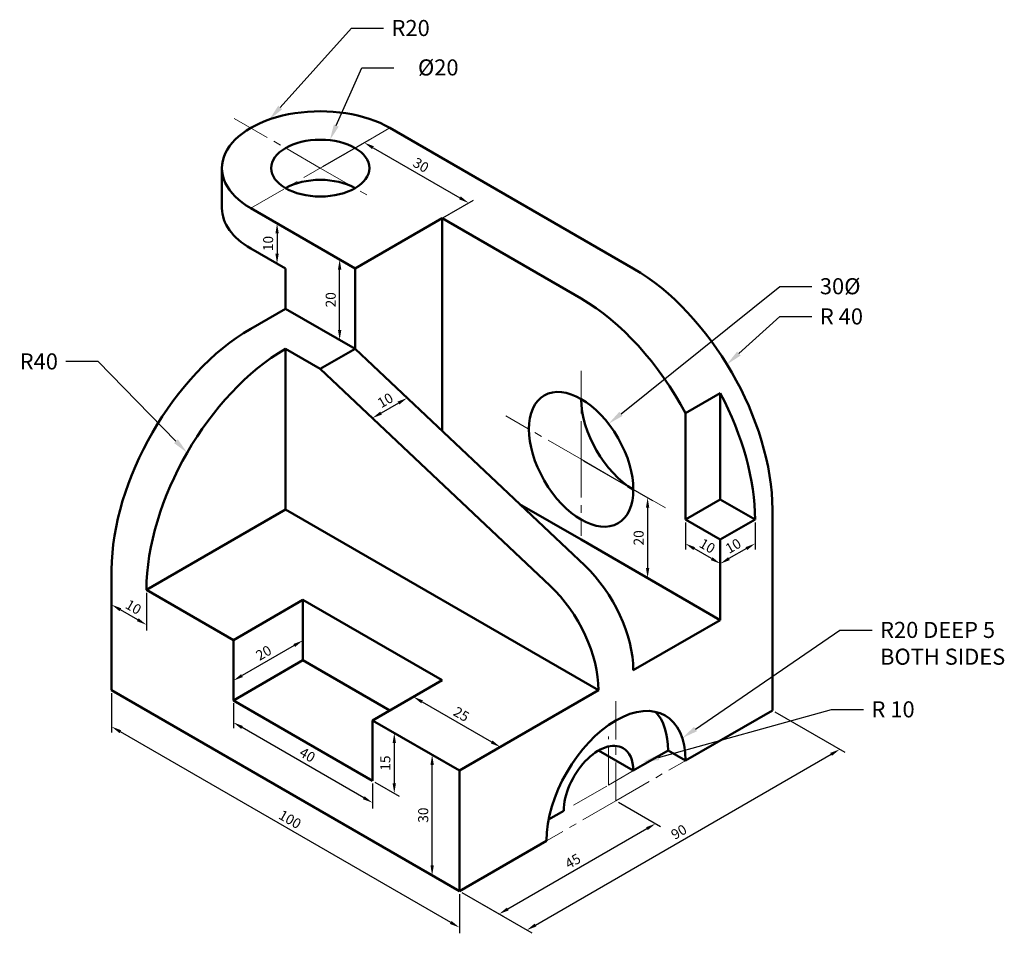
# Model space of a CAD drawing. Units: millimetres. Extents: x 1794 to 2039, y 1624 to 1851.
import ezdxf
from ezdxf import colors
from ezdxf.entities.mleader import LeaderData, LeaderLine
from ezdxf.math import Vec2, Vec3

# ---------------------------------------------------------------- set-up
doc = ezdxf.new("R2010")
doc.units = ezdxf.units.MM
doc.linetypes.add('CENTER', pattern=[50.8, 31.75, -6.35, 6.35, -6.35])
for name, color, linetype, lineweight in [('M-CNTR', 1, 'CENTER', 18), ('M-DIMS', 2, 'Continuous', 25), ('M-OUTL', 7, 'Continuous', 50)]:
    doc.layers.add(name, color=color, linetype=linetype, lineweight=lineweight)
doc.styles.get("Standard").update_dxf_attribs({"font": 'arial.ttf'})
doc.dimstyles.new('ISO-25', dxfattribs={"dimtxt": 2.5, "dimasz": 2.5, "dimexe": 1.25, "dimexo": 0.625, "dimtad": 1, "dimtxsty": 'Standard', "dimcen": 2.5, "dimadec": 0, "dimazin": 0, "dimtfac": 1, "dimtmove": 0, "dimatfit": 3, "dimfxl": 1, "dimarcsym": 0})

# ---------------------------------------------------------------- blocks, each defined once
blk = doc.blocks.new('*D1')
at = {"layer": 'Defpoints', "color": 0, "transparency": 16777216}
for p in [(1942.35, 1657.01), (1903.38, 1634.51), (1913.24, 1628.81)]:
    blk.add_point(p, dxfattribs=at)
at = {"layer": 'M-DIMS', "color": 0, "lineweight": -2, "transparency": 16777216}
for p, q in [((1942.97, 1656.65), (1953.46, 1650.59)), ((1950.05, 1650.06), (1915.41, 1630.06)), ((1904, 1634.15), (1914.49, 1628.09))]:
    blk.add_line(p, q, dxfattribs=at)
at = {"layer": 'M-DIMS', "color": 0, "transparency": 16777216}
for points in [[(1949.84, 1650.42), (1950.26, 1649.7), (1952.21, 1651.31)], [(1915.2, 1630.42), (1915.62, 1629.7), (1913.24, 1628.81)]]:
    blk.add_solid(points, dxfattribs=at)
at = {"layer": 'M-DIMS', "color": 0, "transparency": 16777216, "insert": (1931.78, 1641.71), "char_height": 2.5, "attachment_point": 5, "rotation": 30}
blk.add_mtext('45', dxfattribs=at)
blk = doc.blocks.new('*D2')
at = {"layer": 'Defpoints', "color": 0, "transparency": 16777216}
for p in [(1816.77, 1684.51), (1816.77, 1675.46), (1903.38, 1634.51)]:
    blk.add_point(p, dxfattribs=at)
at = {"layer": 'M-DIMS', "color": 0, "lineweight": -2, "transparency": 16777216}
for p, q in [((1816.77, 1683.79), (1816.77, 1674.01)), ((1901.21, 1626.71), (1818.94, 1674.21)), ((1903.38, 1633.79), (1903.38, 1624.01))]:
    blk.add_line(p, q, dxfattribs=at)
at = {"layer": 'M-DIMS', "color": 0, "transparency": 16777216}
for points in [[(1819.15, 1674.57), (1818.73, 1673.85), (1816.77, 1675.46)], [(1901.42, 1627.07), (1901, 1626.35), (1903.38, 1625.46)]]:
    blk.add_solid(points, dxfattribs=at)
at = {"layer": 'M-DIMS', "color": 0, "transparency": 16777216, "insert": (1861.03, 1652.1), "char_height": 2.5, "attachment_point": 5, "rotation": 330}
blk.add_mtext('100', dxfattribs=at)
blk = doc.blocks.new('*D3')
at = {"layer": 'Defpoints', "color": 0, "transparency": 16777216}
for p in [(1881.73, 1677.01), (1881.73, 1662.01), (1887.15, 1658.88)]:
    blk.add_point(p, dxfattribs=at)
at = {"layer": 'M-DIMS', "color": 0, "lineweight": -2, "transparency": 16777216}
for p, q in [((1882.35, 1676.65), (1888.4, 1673.16)), ((1887.15, 1671.38), (1887.15, 1661.38)), ((1882.35, 1661.65), (1888.4, 1658.16))]:
    blk.add_line(p, q, dxfattribs=at)
at = {"layer": 'M-DIMS', "color": 0, "transparency": 16777216}
for points in [[(1886.73, 1671.38), (1887.57, 1671.38), (1887.15, 1673.88)], [(1886.73, 1661.38), (1887.57, 1661.38), (1887.15, 1658.88)]]:
    blk.add_solid(points, dxfattribs=at)
at = {"layer": 'M-DIMS', "color": 0, "transparency": 16777216, "insert": (1885.25, 1666.38), "char_height": 2.5, "attachment_point": 5, "rotation": 90}
blk.add_mtext('15', dxfattribs=at)
blk = doc.blocks.new('*D4')
at = {"layer": 'Defpoints', "color": 0, "transparency": 16777216}
for p in [(1847.08, 1682.01), (1847.08, 1676.51), (1881.73, 1662.01)]:
    blk.add_point(p, dxfattribs=at)
at = {"layer": 'M-DIMS', "color": 0, "lineweight": -2, "transparency": 16777216}
for p, q in [((1847.08, 1681.29), (1847.08, 1675.07)), ((1879.56, 1657.76), (1849.25, 1675.26)), ((1881.73, 1661.29), (1881.73, 1655.07))]:
    blk.add_line(p, q, dxfattribs=at)
at = {"layer": 'M-DIMS', "color": 0, "transparency": 16777216}
for points in [[(1849.46, 1675.62), (1849.04, 1674.9), (1847.08, 1676.51)], [(1879.77, 1658.12), (1879.35, 1657.4), (1881.73, 1656.51)]]:
    blk.add_solid(points, dxfattribs=at)
at = {"layer": 'M-DIMS', "color": 0, "transparency": 16777216, "insert": (1865.36, 1668.16), "char_height": 2.5, "attachment_point": 5, "rotation": 330}
blk.add_mtext('40', dxfattribs=at)
blk = doc.blocks.new('*D5')
at = {"layer": 'Defpoints', "color": 0, "transparency": 16777216}
for p in [(1981.32, 1679.51), (1998.1, 1669.82), (1903.38, 1634.51)]:
    blk.add_point(p, dxfattribs=at)
at = {"layer": 'M-DIMS', "color": 0, "lineweight": -2, "transparency": 16777216}
for p, q in [((1981.94, 1679.15), (1999.35, 1669.1)), ((1922.32, 1626.07), (1995.93, 1668.57)), ((1904, 1634.15), (1921.4, 1624.1))]:
    blk.add_line(p, q, dxfattribs=at)
at = {"layer": 'M-DIMS', "color": 0, "transparency": 16777216}
for points in [[(1995.72, 1668.93), (1996.14, 1668.21), (1998.1, 1669.82)], [(1922.11, 1626.43), (1922.53, 1625.71), (1920.15, 1624.82)]]:
    blk.add_solid(points, dxfattribs=at)
at = {"layer": 'M-DIMS', "color": 0, "transparency": 16777216, "insert": (1958.18, 1648.97), "char_height": 2.5, "attachment_point": 5, "rotation": 30}
blk.add_mtext('90', dxfattribs=at)
blk = doc.blocks.new('*D6')
at = {"layer": 'Defpoints', "color": 0, "transparency": 16777216}
for p in [(1873.55, 1791.73), (1877.4, 1789.51), (1877.4, 1769.51)]:
    blk.add_point(p, dxfattribs=at)
at = {"layer": 'M-DIMS', "color": 0, "lineweight": -2, "transparency": 16777216}
for p, q in [((1876.77, 1789.87), (1872.3, 1792.45)), ((1873.55, 1774.23), (1873.55, 1789.23)), ((1876.77, 1769.87), (1872.3, 1772.45))]:
    blk.add_line(p, q, dxfattribs=at)
at = {"layer": 'M-DIMS', "color": 0, "transparency": 16777216}
for points in [[(1873.13, 1789.23), (1873.97, 1789.23), (1873.55, 1791.73)], [(1873.13, 1774.23), (1873.97, 1774.23), (1873.55, 1771.73)]]:
    blk.add_solid(points, dxfattribs=at)
at = {"layer": 'M-DIMS', "color": 0, "transparency": 16777216, "insert": (1871.65, 1781.73), "char_height": 2.5, "attachment_point": 5, "rotation": 90}
blk.add_mtext('20', dxfattribs=at)
blk = doc.blocks.new('*D7')
at = {"layer": 'Defpoints', "color": 0, "transparency": 16777216}
for p in [(1877.4, 1769.51), (1868.74, 1764.51), (1881.7, 1752.28)]:
    blk.add_point(p, dxfattribs=at)
at = {"layer": 'M-DIMS', "color": 0, "lineweight": -2, "transparency": 16777216}
for p, q in [((1877.87, 1769.06), (1891.31, 1756.38)), ((1869.21, 1764.06), (1882.65, 1751.38)), ((1888.2, 1756.03), (1883.87, 1753.53))]:
    blk.add_line(p, q, dxfattribs=at)
at = {"layer": 'M-DIMS', "color": 0, "transparency": 16777216}
for points in [[(1887.99, 1756.39), (1888.41, 1755.66), (1890.36, 1757.28)], [(1883.66, 1753.89), (1884.08, 1753.16), (1881.7, 1752.28)]]:
    blk.add_solid(points, dxfattribs=at)
at = {"layer": 'M-DIMS', "color": 0, "transparency": 16777216, "insert": (1885.08, 1756.42), "char_height": 2.5, "attachment_point": 5, "rotation": 30}
blk.add_mtext('10', dxfattribs=at)
blk = doc.blocks.new('*D8')
at = {"layer": 'Defpoints', "color": 0, "transparency": 16777216}
for p in [(1851.41, 1804.51), (1851.41, 1794.51), (1857.97, 1790.73)]:
    blk.add_point(p, dxfattribs=at)
at = {"layer": 'M-DIMS', "color": 0, "lineweight": -2, "transparency": 16777216}
for p, q in [((1852.04, 1804.15), (1859.22, 1800)), ((1857.97, 1798.23), (1857.97, 1793.23)), ((1852.04, 1794.15), (1859.22, 1790))]:
    blk.add_line(p, q, dxfattribs=at)
at = {"layer": 'M-DIMS', "color": 0, "transparency": 16777216}
for points in [[(1857.55, 1798.23), (1858.39, 1798.23), (1857.97, 1800.73)], [(1857.55, 1793.23), (1858.39, 1793.23), (1857.97, 1790.73)]]:
    blk.add_solid(points, dxfattribs=at)
at = {"layer": 'M-DIMS', "color": 0, "transparency": 16777216, "insert": (1856.07, 1795.73), "char_height": 2.5, "attachment_point": 5, "rotation": 90}
blk.add_mtext('10', dxfattribs=at)
blk = doc.blocks.new('*D9')
at = {"layer": 'Defpoints', "color": 0, "transparency": 16777216}
for p in [(1816.77, 1714.51), (1825.43, 1709.51), (1816.77, 1705.82)]:
    blk.add_point(p, dxfattribs=at)
at = {"layer": 'M-DIMS', "color": 0, "lineweight": -2, "transparency": 16777216}
for p, q in [((1816.77, 1713.79), (1816.77, 1704.37)), ((1825.43, 1708.79), (1825.43, 1699.37)), ((1823.27, 1702.07), (1818.94, 1704.57))]:
    blk.add_line(p, q, dxfattribs=at)
at = {"layer": 'M-DIMS', "color": 0, "transparency": 16777216}
for points in [[(1819.15, 1704.93), (1818.73, 1704.21), (1816.77, 1705.82)], [(1823.48, 1702.43), (1823.06, 1701.71), (1825.43, 1700.82)]]:
    blk.add_solid(points, dxfattribs=at)
at = {"layer": 'M-DIMS', "color": 0, "transparency": 16777216, "insert": (1822.05, 1704.96), "char_height": 2.5, "attachment_point": 5, "rotation": 330}
blk.add_mtext('10', dxfattribs=at)
blk = doc.blocks.new('*D10')
at = {"layer": 'Defpoints', "color": 0, "transparency": 16777216}
for p in [(1933.69, 1742.01), (1933.69, 1722.01), (1950.23, 1712.46)]:
    blk.add_point(p, dxfattribs=at)
at = {"layer": 'M-DIMS', "color": 0, "lineweight": -2, "transparency": 16777216}
for p, q in [((1934.31, 1741.65), (1951.48, 1731.74)), ((1950.23, 1729.96), (1950.23, 1714.96)), ((1934.31, 1721.65), (1951.48, 1711.74))]:
    blk.add_line(p, q, dxfattribs=at)
at = {"layer": 'M-DIMS', "color": 0, "transparency": 16777216}
for points in [[(1949.82, 1729.96), (1950.65, 1729.96), (1950.23, 1732.46)], [(1949.82, 1714.96), (1950.65, 1714.96), (1950.23, 1712.46)]]:
    blk.add_solid(points, dxfattribs=at)
at = {"layer": 'M-DIMS', "color": 0, "transparency": 16777216, "insert": (1948.33, 1722.46), "char_height": 2.5, "attachment_point": 5, "rotation": 90}
blk.add_mtext('20', dxfattribs=at)
blk = doc.blocks.new('*D11')
at = {"layer": 'Defpoints', "color": 0, "transparency": 16777216}
for p in [(1959.67, 1727.01), (1968.33, 1722.01), (1959.67, 1721.03)]:
    blk.add_point(p, dxfattribs=at)
at = {"layer": 'M-DIMS', "color": 0, "lineweight": -2, "transparency": 16777216}
for p, q in [((1959.67, 1726.29), (1959.67, 1719.59)), ((1968.33, 1721.29), (1968.33, 1714.59)), ((1966.16, 1717.28), (1961.83, 1719.78))]:
    blk.add_line(p, q, dxfattribs=at)
at = {"layer": 'M-DIMS', "color": 0, "transparency": 16777216}
for points in [[(1962.04, 1720.14), (1961.62, 1719.42), (1959.67, 1721.03)], [(1966.37, 1717.64), (1965.95, 1716.92), (1968.33, 1716.03)]]:
    blk.add_solid(points, dxfattribs=at)
at = {"layer": 'M-DIMS', "color": 0, "transparency": 16777216, "insert": (1964.95, 1720.18), "char_height": 2.5, "attachment_point": 5, "rotation": 330}
blk.add_mtext('10', dxfattribs=at)
blk = doc.blocks.new('*D12')
at = {"layer": 'Defpoints', "color": 0, "transparency": 16777216}
for p in [(1976.99, 1727.01), (1968.33, 1722.01), (1968.33, 1716.03)]:
    blk.add_point(p, dxfattribs=at)
at = {"layer": 'M-DIMS', "color": 0, "lineweight": -2, "transparency": 16777216}
for p, q in [((1976.99, 1726.29), (1976.99, 1719.59)), ((1968.33, 1721.29), (1968.33, 1714.59)), ((1974.82, 1719.78), (1970.49, 1717.28))]:
    blk.add_line(p, q, dxfattribs=at)
at = {"layer": 'M-DIMS', "color": 0, "transparency": 16777216}
for points in [[(1974.61, 1720.14), (1975.03, 1719.42), (1976.99, 1721.03)], [(1970.28, 1717.64), (1970.7, 1716.92), (1968.33, 1716.03)]]:
    blk.add_solid(points, dxfattribs=at)
at = {"layer": 'M-DIMS', "color": 0, "transparency": 16777216, "insert": (1971.71, 1720.18), "char_height": 2.5, "attachment_point": 5, "rotation": 30}
blk.add_mtext('10', dxfattribs=at)
blk = doc.blocks.new('*D13')
at = {"layer": 'Defpoints', "color": 0, "transparency": 16777216}
for p in [(1896.58, 1668.43), (1903.38, 1664.51), (1903.38, 1634.51)]:
    blk.add_point(p, dxfattribs=at)
at = {"layer": 'M-DIMS', "color": 0, "lineweight": -2, "transparency": 16777216}
for p, q in [((1902.75, 1664.87), (1895.33, 1669.15)), ((1896.58, 1640.93), (1896.58, 1665.93)), ((1902.75, 1634.87), (1895.33, 1639.15))]:
    blk.add_line(p, q, dxfattribs=at)
at = {"layer": 'M-DIMS', "color": 0, "transparency": 16777216}
for points in [[(1896.17, 1665.93), (1897, 1665.93), (1896.58, 1668.43)], [(1896.17, 1640.93), (1897, 1640.93), (1896.58, 1638.43)]]:
    blk.add_solid(points, dxfattribs=at)
at = {"layer": 'M-DIMS', "color": 0, "transparency": 16777216, "insert": (1894.68, 1653.43), "char_height": 2.5, "attachment_point": 5, "rotation": 90}
blk.add_mtext('30', dxfattribs=at)
blk = doc.blocks.new('*D14')
at = {"layer": 'Defpoints', "color": 0, "transparency": 16777216}
for p in [(1864.4, 1692.01), (1847.08, 1686.92), (1847.08, 1682.01)]:
    blk.add_point(p, dxfattribs=at)
at = {"layer": 'M-DIMS', "color": 0, "lineweight": -2, "transparency": 16777216}
for p, q in [((1864.4, 1692.73), (1864.4, 1698.36)), ((1862.24, 1695.67), (1849.25, 1688.17)), ((1847.08, 1682.73), (1847.08, 1688.36))]:
    blk.add_line(p, q, dxfattribs=at)
at = {"layer": 'M-DIMS', "color": 0, "transparency": 16777216}
for points in [[(1862.03, 1696.03), (1862.45, 1695.31), (1864.4, 1696.92)], [(1849.04, 1688.53), (1849.46, 1687.81), (1847.08, 1686.92)]]:
    blk.add_solid(points, dxfattribs=at)
at = {"layer": 'M-DIMS', "color": 0, "transparency": 16777216, "insert": (1854.79, 1693.56), "char_height": 2.5, "attachment_point": 5, "rotation": 30}
blk.add_mtext('20', dxfattribs=at)
blk = doc.blocks.new('*D15')
at = {"layer": 'Defpoints', "color": 0, "transparency": 16777216}
for p in [(1881.73, 1677.01), (1913.56, 1670.39), (1903.38, 1664.51)]:
    blk.add_point(p, dxfattribs=at)
at = {"layer": 'M-DIMS', "color": 0, "lineweight": -2, "transparency": 16777216}
for p, q in [((1882.35, 1677.37), (1893.16, 1683.61)), ((1894.08, 1681.64), (1911.4, 1671.64)), ((1904, 1664.87), (1914.81, 1671.11))]:
    blk.add_line(p, q, dxfattribs=at)
at = {"layer": 'M-DIMS', "color": 0, "transparency": 16777216}
for points in [[(1894.29, 1682), (1893.87, 1681.28), (1891.91, 1682.89)], [(1911.61, 1672), (1911.19, 1671.28), (1913.56, 1670.39)]]:
    blk.add_solid(points, dxfattribs=at)
at = {"layer": 'M-DIMS', "color": 0, "transparency": 16777216, "insert": (1903.69, 1678.29), "char_height": 2.5, "attachment_point": 5, "rotation": 330}
blk.add_mtext('25', dxfattribs=at)
blk = doc.blocks.new('*D16')
at = {"layer": 'Defpoints', "color": 0, "transparency": 16777216}
for p in [(1868.74, 1814.51), (1905.67, 1805.84), (1894.72, 1799.51)]:
    blk.add_point(p, dxfattribs=at)
at = {"layer": 'M-DIMS', "color": 0, "lineweight": -2, "transparency": 16777216}
for p, q in [((1869.36, 1814.87), (1880.94, 1821.56)), ((1881.86, 1819.59), (1903.51, 1807.09)), ((1895.34, 1799.87), (1906.92, 1806.56))]:
    blk.add_line(p, q, dxfattribs=at)
at = {"layer": 'M-DIMS', "color": 0, "transparency": 16777216}
for points in [[(1882.07, 1819.95), (1881.65, 1819.23), (1879.69, 1820.84)], [(1903.72, 1807.45), (1903.3, 1806.73), (1905.67, 1805.84)]]:
    blk.add_solid(points, dxfattribs=at)
at = {"layer": 'M-DIMS', "color": 0, "transparency": 16777216, "insert": (1893.63, 1814.98), "char_height": 2.5, "attachment_point": 5, "rotation": 330}
blk.add_mtext('30', dxfattribs=at)

msp = doc.modelspace()

# ---------------------------------------------------------------- linework, layer by layer
at = {"layer": 'M-CNTR', "ltscale": 0.3}
for p, q in [((1868.735, 1814.51), (1846.545, 1827.322)), ((1851.415, 1804.51), (1886.056, 1824.51)), ((1868.735, 1814.51), (1880.726, 1807.587)), ((1933.687, 1742.01), (1933.687, 1764.025)), ((1933.687, 1742.01), (1914.957, 1752.823)), ((1933.687, 1742.01), (1954.669, 1729.896)), ((1933.687, 1742.01), (1933.687, 1722.935)), ((1942.347, 1657.01), (1942.347, 1682.595)), ((1940.457, 1660.919), (1940.457, 1673.015)), ((1940.457, 1660.919), (1949.117, 1665.919)), ((1942.347, 1657.01), (1959.907, 1667.148)), ((1931.797, 1655.919), (1940.457, 1660.919)), ((1942.347, 1657.01), (1924.094, 1646.471))]:
    msp.add_line(p, q, dxfattribs=at)
at = {"layer": 'M-OUTL'}
for p, q in [((1946.677, 1789.51), (1886.056, 1824.51)), ((1844.24, 1814.51), (1844.24, 1804.51)), ((1877.395, 1789.51), (1851.415, 1804.51)), ((1877.395, 1789.51), (1899.046, 1802.01)), ((1933.687, 1782.01), (1899.046, 1802.01)), ((1899.046, 1802.01), (1899.046, 1749.085)), ((1851.415, 1794.51), (1860.075, 1789.51)), ((1860.075, 1789.51), (1860.075, 1779.51)), ((1877.395, 1769.51), (1877.395, 1789.51)), ((1851.415, 1774.51), (1860.075, 1779.51)), ((1860.075, 1779.51), (1877.395, 1769.51)), ((1860.075, 1729.51), (1860.075, 1769.51)), ((1868.735, 1764.51), (1860.075, 1769.51)), ((1877.395, 1769.51), (1868.735, 1764.51)), ((1934.591, 1715.553), (1877.395, 1769.51)), ((1925.93, 1710.553), (1868.735, 1764.51)), ((1959.668, 1753.467), (1968.328, 1758.467)), ((1968.328, 1758.467), (1968.328, 1732.01)), ((1959.668, 1727.01), (1959.668, 1753.467)), ((1968.328, 1732.01), (1959.668, 1727.01)), ((1976.988, 1727.01), (1968.328, 1732.01)), ((1825.434, 1709.51), (1860.075, 1729.51)), ((1860.075, 1729.51), (1938.017, 1684.51)), ((1933.687, 1722.01), (1918.376, 1730.85)), ((1981.318, 1709.51), (1981.318, 1729.51)), ((1959.668, 1727.01), (1968.328, 1722.01)), ((1968.328, 1722.01), (1976.988, 1727.01)), ((1968.328, 1702.01), (1933.687, 1722.01)), ((1968.328, 1702.01), (1968.328, 1722.01)), ((1816.774, 1714.51), (1816.774, 1684.51)), ((1847.084, 1697.01), (1825.434, 1709.51)), ((1981.318, 1679.51), (1981.318, 1709.51)), ((1864.405, 1707.01), (1847.084, 1697.01)), ((1899.046, 1687.01), (1864.405, 1707.01)), ((1864.405, 1692.01), (1864.405, 1707.01)), ((1946.677, 1689.51), (1968.328, 1702.01)), ((1847.084, 1682.01), (1847.084, 1697.01)), ((1847.084, 1682.01), (1864.405, 1692.01)), ((1864.405, 1692.01), (1886.056, 1679.51)), ((1881.725, 1677.01), (1899.046, 1687.01)), ((1816.774, 1684.51), (1903.376, 1634.51)), ((1903.376, 1664.51), (1938.017, 1684.51)), ((1881.725, 1662.01), (1847.084, 1682.01)), ((1959.668, 1667.01), (1981.318, 1679.51)), ((1903.376, 1664.51), (1881.725, 1677.01)), ((1881.725, 1677.01), (1881.725, 1662.01)), ((1946.677, 1664.51), (1938.017, 1669.51)), ((1955.338, 1669.51), (1946.677, 1664.51)), ((1949.117, 1665.919), (1955.338, 1669.51)), ((1959.668, 1667.01), (1955.338, 1669.51)), ((1903.376, 1634.51), (1903.376, 1664.51)), ((1929.357, 1654.51), (1925.577, 1652.327)), ((1903.376, 1634.51), (1925.027, 1647.01))]:
    msp.add_line(p, q, dxfattribs=at)
for centre, major_axis, start_param, end_param in [((1868.735, 1814.51), (-24.495, 0), 3.9269908, 7.0685835), ((1868.735, 1804.51), (12.247, 0), 0.7853982, 2.3561945), ((1868.735, 1804.51), (-24.495, 0), 0, 0.7853982), ((1946.677, 1749.51), (24.495, -42.426), 7.0685835, 8.6393798), ((1933.687, 1742.01), (24.495, -42.426), 1.5081324, 2.3561945), ((1851.415, 1734.51), (-24.495, -42.426), 3.9269908, 5.4977871), ((1860.075, 1729.51), (-24.495, -42.426), 3.9269908, 5.4977871), ((1942.347, 1747.01), (24.495, -42.426), 7.0685835, 7.7913177), ((1946.677, 1749.51), (9.186, -15.91), 3.9269908, 5.4977871), ((1929.357, 1699.51), (12.247, -21.213), 7.0685835, 8.3324121), ((1920.697, 1694.51), (12.247, -21.213), 7.0685835, 8.3324121), ((1942.347, 1657.01), (-12.247, -21.213), 2.3561945, 5.4977871), ((1938.017, 1659.51), (-12.247, -21.213), 8.6393798, 9.2470674), ((1938.017, 1659.51), (-6.124, -10.607), 3.1415927, 5.4977871), ((1938.017, 1659.51), (-6.124, -10.607), 2.3561945, 3.1415927)]:
    msp.add_ellipse(centre, major_axis=major_axis, ratio=0.5773503, start_param=start_param, end_param=end_param, dxfattribs=at)
for centre, major_axis in [((1868.735, 1814.51), (-12.247, 0)), ((1933.687, 1742.01), (9.186, -15.91))]:
    msp.add_ellipse(centre, major_axis=major_axis, ratio=0.5773503, dxfattribs=at)

# ---------------------------------------------------------------- dimensions: what is measured, and where the dimension line sits
at = {"layer": 'M-DIMS'}
for p1, p2, distance, picture, middle in [((1868.735, 1814.51), (1894.716, 1799.51), 10.958, '*D16', (1893.635, 1814.984)), ((1851.415, 1804.51), (1851.415, 1794.51), 6.554, '*D8', (1856.067, 1795.726)), ((1877.395, 1769.51), (1877.395, 1789.51), 3.844, '*D6', (1871.649, 1781.73)), ((1877.395, 1769.51), (1868.735, 1764.51), 17.08, '*D7', (1885.084, 1756.422)), ((1933.687, 1742.01), (1933.687, 1722.01), 16.545, '*D10', (1948.331, 1722.457)), ((1968.328, 1722.01), (1959.668, 1727.01), 5.178, '*D11', (1964.949, 1720.177)), ((1976.988, 1727.01), (1968.328, 1722.01), 5.178, '*D12', (1971.707, 1720.177)), ((1825.434, 1709.51), (1816.774, 1714.51), 7.527, '*D9', (1822.054, 1704.965)), ((1864.405, 1692.01), (1847.084, 1682.01), -4.249, '*D14', (1854.794, 1693.563)), ((1903.376, 1634.51), (1816.774, 1684.51), 7.84, '*D2', (1861.025, 1652.104)), ((1881.725, 1662.01), (1847.084, 1682.01), 4.762, '*D4', (1865.356, 1668.158)), ((1881.725, 1677.01), (1903.376, 1664.51), 10.189, '*D15', (1903.69, 1678.289)), ((1903.376, 1634.51), (1981.318, 1679.51), -16.779, '*D5', (1958.175, 1648.969)), ((1881.725, 1677.01), (1881.725, 1662.01), 5.424, '*D3', (1885.248, 1666.378)), ((1903.376, 1634.51), (1903.376, 1664.51), 6.794, '*D13', (1894.68, 1653.432)), ((1942.347, 1657.01), (1903.376, 1634.51), 9.867, '*D1', (1931.781, 1641.705))]:
    dim = msp.add_aligned_dim(p1=p1, p2=p2, distance=distance, dimstyle='ISO-25', override={"dimclrd": 0, "dimclre": 0, "dimclrt": 0}, dxfattribs=at)
    dim.commit()
    dim.dimension.update_dxf_attribs({"geometry": picture, "text_midpoint": middle})

# ---------------------------------------------------------------- leaders
ml = msp.add_multileader_mtext('Standard', dxfattribs=at)
ml.set_content('R20', color=256)
ml.set_leader_properties()
ml.build(insert=Vec2(0, 0))
ctx = ml.context
ctx.base_point, ctx.plane_origin = Vec3(1884.469, 1849.351), Vec3(1856.068, 1826.614)
notes = []
notes.append((ctx, [(0, (1, 1, 0), (1876.469, 1849.351), (1, 0), 8, [(0, [(1856.068, 1826.614)], 0, [])])]))
ctx.mtext.insert, ctx.mtext.flow_direction = Vec3(1886.469, 1851.385), 5
ml = msp.add_multileader_mtext('Standard', dxfattribs=at)
ml.set_content('\\pxi-3,l4,t4;%%C20', color=256)
ml.set_leader_properties()
ml.build(insert=Vec2(0, 0))
ctx = ml.context
ctx.base_point, ctx.plane_origin = Vec3(1887.054, 1839.493), Vec3(1871.102, 1821.448)
notes.append((ctx, [(0, (1, 1, 0), (1879.054, 1839.493), (1, 0), 8, [(0, [(1871.102, 1821.448)], 0, [])])]))
ctx.mtext.insert, ctx.mtext.flow_direction = Vec3(1889.054, 1841.573), 5
ml = msp.add_multileader_mtext('Standard', dxfattribs=at)
ml.set_content('30%%C', color=256)
ml.set_leader_properties()
ml.build(insert=Vec2(0, 0))
ctx = ml.context
ctx.base_point, ctx.plane_origin = Vec3(1991.126, 1785.019), Vec3(1940.502, 1750.846)
notes.append((ctx, [(0, (1, 1, 0), (1983.126, 1785.019), (1, 0), 8, [(0, [(1940.502, 1750.846)], 0, [])])]))
ctx.mtext.insert, ctx.mtext.flow_direction = Vec3(1993.126, 1787.099), 5
ml = msp.add_multileader_mtext('Standard', dxfattribs=at)
ml.set_content('R 40', color=256)
ml.set_leader_properties()
ml.build(insert=Vec2(0, 0))
ctx = ml.context
ctx.base_point, ctx.plane_origin = Vec3(1991.126, 1777.552), Vec3(1969.986, 1765.643)
notes.append((ctx, [(0, (1, 1, 0), (1983.126, 1777.552), (1, 0), 8, [(0, [(1969.986, 1765.643)], 0, [])])]))
ctx.mtext.insert, ctx.mtext.flow_direction = Vec3(1993.126, 1779.587), 5
ml = msp.add_multileader_mtext('Standard', dxfattribs=at)
ml.set_content('R40', color=256)
ml.set_leader_properties()
ml.build(insert=Vec2(0, 0))
ctx = ml.context
ctx.base_point, ctx.plane_origin = Vec3(1791.857, 1766.355), Vec3(1835.58, 1743.652)
ctx.text_align_type = 2
notes.append((ctx, [(0, (1, 1, 0), (1813.402, 1766.355), (-1, 0), 8, [(0, [(1835.58, 1743.652)], 0, [])])]))
ctx.mtext.insert, ctx.mtext.alignment, ctx.mtext.flow_direction = Vec3(1803.402, 1768.389), 3, 5
ml = msp.add_multileader_mtext('Standard', dxfattribs=at)
ml.set_content('R20 DEEP 5\\PBOTH SIDES', color=256)
ml.set_leader_properties()
ml.build(insert=Vec2(0, 0))
ctx = ml.context
ctx.base_point, ctx.plane_origin = Vec3(2006.12, 1699.51), Vec3(1958.852, 1672.604)
notes.append((ctx, [(0, (1, 1, 0), (1998.12, 1699.51), (1, 0), 8, [(0, [(1958.852, 1672.604)], 0, [])])]))
ctx.mtext.insert, ctx.mtext.flow_direction = Vec3(2008.12, 1701.544), 5
ml = msp.add_multileader_mtext('Standard', dxfattribs=at)
ml.set_content('R 10', color=256)
ml.set_leader_properties()
ml.build(insert=Vec2(0, 0))
ctx = ml.context
ctx.base_point, ctx.plane_origin = Vec3(2003.986, 1679.733), Vec3(1949.089, 1666.705)
notes.append((ctx, [(0, (1, 1, 0), (1995.986, 1679.733), (1, 0), 8, [(0, [(1949.089, 1666.705)], 0, [])])]))
ctx.mtext.insert, ctx.mtext.flow_direction = Vec3(2005.986, 1681.768), 5
for ctx, leaders in notes:
    for number, flags, end, landing, length, lines in leaders:
        leader = LeaderData()
        leader.index, (leader.has_last_leader_line, leader.has_dogleg_vector, leader.attachment_direction) = number, flags
        leader.last_leader_point, leader.dogleg_vector, leader.dogleg_length = Vec3(end), Vec3(landing), length
        for number, points, colour, breaks in lines:
            line = LeaderLine()
            line.index, line.vertices, line.color, line.breaks = number, Vec3.list(points), colors.encode_raw_color(colour), breaks
            leader.lines.append(line)
        ctx.leaders.append(leader)

doc.saveas('drawing.dxf')
